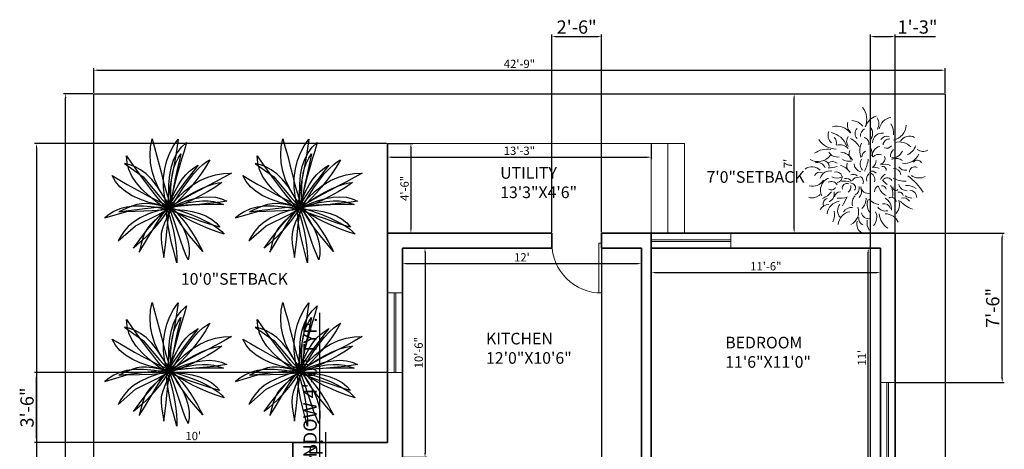
# Model space of a CAD drawing. Units: inches. Extents: x 3394 to 4794, y 965 to 1718.
# Tile 15 of 15: x 4177 to 4770, y 1453 to 1711. Entities that reach past the tile are written whole.
import ezdxf

# ---------------------------------------------------------------- set-up
doc = ezdxf.new("R2010")
doc.units = ezdxf.units.IN
for name, color, linetype, lineweight in [('A-ANNO-DIMS', 2, 'Continuous', 13), ('A-ANNO-TEXT', 7, 'Continuous', 18), ('A-AREA-IDEN', 7, 'Continuous', 18), ('A-DOOR', 4, 'Continuous', 18), ('A-FLOR', 7, 'Continuous', 18), ('A-FLOR-STRS', 7, 'Continuous', 18), ('A-GLAZ', 4, 'Continuous', 18), ('A-WALL', 7, 'Continuous', 35), ('C-PROP', 7, 'Continuous', 25), ('CAY', 94, 'Continuous', 13)]:
    doc.layers.add(name, color=color, linetype=linetype, lineweight=lineweight)
doc.layers.add('DIENHOA', color=3, linetype='Continuous')
doc.styles.add('ATT', font='romans.shx')
doc.styles.get("Standard").update_dxf_attribs({"font": 'arial.ttf'})
doc.dimstyles.new('ISO-25', dxfattribs={"dimtxt": 8, "dimasz": 2.5, "dimexe": 1.25, "dimexo": 0.625, "dimtad": 1, "dimlunit": 3, "dimtxsty": 'Standard', "dimcen": 2.5, "dimadec": 0, "dimazin": 0, "dimtfac": 1, "dimtmove": 0, "dimatfit": 3, "dimfxl": 1, "dimarcsym": 0})

# ---------------------------------------------------------------- blocks, each defined once
blk = doc.blocks.new('*U5')
for p, q in [((0, 0), (0, -6)), ((30, 0), (30, -6))]:
    blk.add_line(p, q)
blk.add_lwpolyline([(0, 0), (0, 30), (1.75, 30), (1.75, 0)], close=True)
blk.add_arc((0, 0), 30, 0, 90)
blk = doc.blocks.new('Cay03_mb')
at = {"layer": 'DIENHOA'}
for p, q in [((79.5, 503.7), (118.6, 555.3)), ((118.6, 555.3), (166.2, 599.1)), ((166.2, 599.1), (142.2, 519.4)), ((48.6, 443.6), (79.5, 503.7)), ((142.2, 519.4), (119, 441.7)), ((-365.2, 390.3), (-414.4, 402.8)), ((-414.4, 402.8), (-240.2, 277.8)), ((-314.9, 371.3), (-365.2, 390.3)), ((-263.5, 343.5), (-314.9, 371.3)), ((9.9, 295.3), (25.5, 374.3)), ((25.5, 374.3), (48.6, 443.6)), ((119, 441.7), (96.7, 365.6)), ((-211.2, 304.6), (-263.5, 343.5)), ((-240.2, 277.8), (-88.4, 94.9)), ((-158, 252.3), (-211.2, 304.6)), ((1.6, 205.7), (9.9, 295.3)), ((75.6, 290.6), (55.7, 216.3)), ((96.7, 365.6), (75.6, 290.6)), ((363.4, 275.4), (436.8, 297.2)), ((436.8, 297.2), (511, 309.6)), ((511, 309.6), (585.9, 313.5)), ((585.9, 313.5), (511.8, 271.4)), ((-104.2, 184.4), (-158, 252.3)), ((-49.6, 98.5), (-104.2, 184.4)), ((0.2, 104.9), (1.6, 205.7)), ((55.7, 216.3), (37.3, 142.1)), ((147, 144.1), (218.5, 199.8)), ((218.5, 199.8), (290.6, 243.2)), ((363.7, 192.9), (290.2, 154.9)), ((290.6, 243.2), (363.4, 275.4)), ((437.6, 231.5), (363.7, 192.9)), ((511.8, 271.4), (437.6, 231.5)), ((-88.4, 94.9), (5.4, -7.8)), ((5.4, -7.8), (-49.6, 98.5)), ((5.4, -7.8), (0.2, 104.9)), ((37.3, 142.1), (20.5, 67.6)), ((75.9, 75.2), (147, 144.1)), ((217.4, 116.6), (145.5, 77.3)), ((290.2, 154.9), (217.4, 116.6)), ((-345, 5.4), (-399.6, -17.1)), ((-298.6, 20.1), (-345, 5.4)), ((-254.7, 27.4), (-298.6, 20.1)), ((-208, 27.8), (-254.7, 27.4)), ((-152.7, 21.7), (-208, 27.8)), ((-83.4, 9.7), (-152.7, 21.7)), ((5.4, -7.8), (-83.4, 9.7)), ((5.4, -7.8), (75.9, 75.2)), ((20.5, 67.6), (5.4, -7.8)), ((74.7, 36.1), (5.4, -7.8)), ((5.4, -7.8), (100.3, 18.4)), ((46.3, 0.9), (5.4, -7.8)), ((96.7, 7.5), (46.3, 0.9)), ((145.5, 77.3), (74.7, 36.1)), ((155, 12.2), (96.7, 7.5)), ((100.3, 18.4), (182.2, 37.2)), ((219.6, 15.4), (155, 12.2)), ((182.2, 37.2), (253, 48.9)), ((289, 17.4), (219.6, 15.4)), ((253, 48.9), (314.6, 54.1)), ((361.6, 18.5), (289, 17.4)), ((314.6, 54.1), (369.2, 53.3)), ((435.8, 18.9), (361.6, 18.5)), ((369.2, 53.3), (418.6, 46.8)), ((418.6, 46.8), (464.9, 35.2)), ((510, 19), (435.8, 18.9)), ((464.9, 35.2), (510, 19)), ((-399.6, -17.1), (-468, -47.9)), ((-468, -47.9), (-375.6, -37.8)), ((-375.6, -37.8), (-295.3, -27.9)), ((-295.3, -27.9), (-225.8, -18.9)), ((-225.8, -18.9), (-165.8, -11.3)), ((-165.8, -11.3), (-114, -5.7)), ((-120.2, -122.1), (-79.8, -79.6)), ((-114, -5.7), (-69, -2.9)), ((-79.8, -79.6), (-45.1, -46.3)), ((-33.2, -69.5), (-74.6, -127.3)), ((-69, -2.9), (-29.6, -3.4)), ((-45.1, -46.3), (-16.5, -22.4)), ((5.4, -7.8), (-33.2, -69.5)), ((-29.6, -3.4), (5.4, -7.8)), ((-16.5, -22.4), (5.4, -7.8)), ((5.4, -7.8), (56.8, -73.3)), ((25.9, -64.4), (5.4, -7.8)), ((5.4, -7.8), (112.8, -40.3)), ((53.5, -41.6), (5.4, -7.8)), ((47, -125.9), (25.9, -64.4)), ((107, -75.7), (53.5, -41.6)), ((56.8, -73.3), (100.4, -139.1)), ((165.5, -109.6), (107, -75.7)), ((112.8, -40.3), (207.5, -73.8)), ((207.5, -73.8), (289.5, -107.6)), ((-216.3, -235.6), (-165.9, -174.1)), ((-165.9, -174.1), (-120.2, -122.1)), ((-117.8, -181.1), (-162.1, -230.9)), ((-74.6, -127.3), (-117.8, -181.1)), ((68.7, -190.6), (47, -125.9)), ((100.4, -139.1), (135.9, -204.3)), ((228.7, -142.8), (165.5, -109.6)), ((296, -174.7), (228.7, -142.8)), ((289.5, -107.6), (359.3, -141.1)), ((367.1, -204.8), (296, -174.7)), ((359.3, -141.1), (416.9, -173.5)), ((416.9, -173.5), (462.6, -204.2)), ((-271, -306.6), (-216.3, -235.6)), ((-162.1, -230.9), (-206.3, -276.5)), ((90.8, -256.6), (68.7, -190.6)), ((113.1, -322.2), (90.8, -256.6)), ((135.9, -204.3), (162.8, -268.3)), ((162.8, -268.3), (181, -330.4)), ((441.6, -232.7), (367.1, -204.8)), ((518.9, -257.7), (441.6, -232.7)), ((462.6, -204.2), (496.5, -232.5)), ((496.5, -232.5), (518.9, -257.7)), ((-329.5, -387.1), (-271, -306.6)), ((-291, -354.7), (-329.5, -387.1)), ((-249.6, -317.8), (-291, -354.7)), ((-206.3, -276.5), (-249.6, -317.8)), ((135.4, -385.6), (113.1, -322.2)), ((181, -330.4), (190, -390)), ((157.6, -445), (135.4, -385.6)), ((179.5, -498.7), (157.6, -445)), ((189.6, -446.3), (179.5, -498.7)), ((190, -390), (189.6, -446.3))]:
    blk.add_line(p, q, dxfattribs=at)
for points in [[(23.7, -5.4), (-41, 82.2), (-91.8, 167.1), (-129.7, 249.5), (-155.6, 329.6), (-170.2, 407.8), (-174.7, 484.2), (-169.8, 559.3), (-156.5, 633.1)], [(-156.5, 633.1), (-132.5, 551.3), (-110.5, 470), (-89.8, 389.2), (-69.6, 309), (-49, 229.4), (-27.1, 150.4), (-3.2, 72.1), (23.7, -5.4)], [(-16.4, -26.7), (-38.3, 80), (-48.9, 178.3), (-48.7, 269), (-38.5, 352.6), (-19.1, 429.7), (9, 501), (44.9, 567.1), (87.9, 628.5)], [(87.9, 628.5), (75.5, 544.2), (61.3, 461.2), (46.1, 379.1), (30.8, 297.8), (16.1, 216.9), (2.9, 136), (-8.3, 54.9), (-16.4, -26.7)], [(-395.6, 473.7), (-347.5, 405.6), (-300.6, 339.5), (-254.3, 275.1), (-208.3, 212.3), (-161.9, 150.9), (-114.8, 90.7), (-66.5, 31.6), (-16.4, -26.7)], [(-16.4, -26.7), (-108.3, 38.6), (-186.9, 101.7), (-252.4, 163.5), (-305.1, 224.4), (-345.4, 285.2), (-373.7, 346.6), (-390.4, 409.2), (-395.6, 473.7)], [(23.7, -5.4), (19.8, 93), (20.3, 177), (25, 248.5), (34, 309.8), (47.3, 362.7), (64.9, 409.3), (86.8, 451.7), (112.9, 491.9)], [(112.9, 491.9), (96, 419.7), (79.5, 347.4), (63.9, 276.5), (50, 208.4), (38.4, 144.8), (29.7, 86.9), (24.6, 36.3), (23.7, -5.4)], [(273.2, 387.3), (227.6, 328.8), (182.3, 270.1), (138.4, 212.3), (97.2, 156.4), (60, 103.4), (27.8, 54.6), (1.9, 10.8), (-16.4, -26.7)], [(-16.4, -26.7), (21.4, 64.2), (57, 140.3), (91.4, 203.3), (125.2, 255.1), (159.5, 297.5), (195, 332.5), (232.7, 361.8), (273.2, 387.3)], [(384.3, 437.5), (342.2, 367.8), (298.1, 301.7), (252.6, 239.4), (206.1, 181.1), (159.4, 127.2), (113, 78), (67.6, 33.6), (23.7, -5.4)], [(23.7, -5.4), (79.9, 91.7), (134.1, 176.2), (185.8, 248.4), (234.3, 308.7), (279, 357.3), (319.3, 394.8), (354.6, 421.4), (384.3, 437.5)], [(-530.5, 289.7), (-458.3, 248.1), (-387.9, 207.8), (-318.9, 168.7), (-250.8, 131.1), (-182.9, 94.8), (-114.9, 59.9), (-46.2, 26.5), (23.7, -5.4)], [(23.7, -5.4), (-87.2, 15.2), (-185, 39.6), (-270.3, 68.2), (-343.7, 101.4), (-405.9, 139.7), (-457.3, 183.5), (-498.7, 233.4), (-530.5, 289.7)], [(496.7, 224), (429.4, 178.4), (361.6, 136.9), (294.1, 99.5), (227.5, 66.1), (162.4, 36.7), (99.7, 11.5), (39.8, -9.7), (-16.4, -26.7)], [(-16.4, -26.7), (75.4, 37.9), (160.1, 91.8), (237.3, 135.7), (306.6, 170), (367.6, 195.4), (419.9, 212.5), (463.1, 221.9), (496.7, 224)], [(-16.4, -26.7), (-134, -4.7), (-235.3, 5.3), (-322, 4.7), (-395.9, -5), (-458.7, -22.3), (-512.3, -45.7), (-558.2, -73.6), (-598.4, -104.7)], [(23.7, -5.4), (99.3, 29.7), (173.2, 57.1), (244.8, 76.7), (313.3, 88.3), (377.9, 91.8), (437.9, 87), (492.7, 73.8), (541.4, 52)], [(541.4, 52), (484.1, 42.9), (421.2, 34.8), (354.4, 27.6), (285.4, 20.9), (216.1, 14.5), (148.2, 8.1), (83.5, 1.6), (23.7, -5.4)], [(-598.4, -104.7), (-392.7, -44.4), (-155, -37.4), (-16.4, -26.7)], [(-471.9, -320.3), (-310.5, -179.3), (-97.7, -73.3), (23.7, -5.4)], [(23.7, -5.4), (-92.3, -34.8), (-188.4, -68.2), (-266.9, -105.1), (-329.9, -144.9), (-379.7, -187), (-418.5, -230.7), (-448.5, -275.3), (-471.9, -320.3)], [(-276.2, -424.4), (-227.3, -345.4), (-185.7, -276.1), (-150, -215.7), (-119.1, -163.8), (-91.5, -119.5), (-66, -82.3), (-41.4, -51.6), (-16.4, -26.7)], [(-16.4, -26.7), (-84.9, -86), (-137, -133.1), (-175.8, -173), (-204.3, -210), (-225.5, -249.1), (-242.5, -294.7), (-258.4, -351.6), (-276.2, -424.4)], [(23.7, -5.4), (-13.6, -87.9), (-41.1, -152.6), (-59.6, -205), (-69.9, -250.7), (-72.8, -295), (-69.2, -343.6), (-59.7, -401.9), (-45.3, -475.5)], [(-45.3, -475.5), (-34.1, -383.2), (-25.4, -302.8), (-18.3, -233.1), (-12, -172.9), (-5.6, -121.2), (2, -76.8), (11.4, -38.5), (23.7, -5.4)], [(76.2, -524.2), (48.8, -428.5), (26.6, -341.7), (9.2, -264.1), (-3.6, -196.1), (-12.3, -138), (-17.1, -90.2), (-18.3, -53), (-16.4, -26.7)], [(-16.4, -26.7), (66.9, -26.6), (145.6, -32.7), (218.8, -44.9), (285.8, -63.1), (345.9, -87.1), (398.4, -116.6), (442.6, -151.6), (477.6, -191.8)], [(477.6, -191.8), (421.8, -176), (361.3, -156.9), (297.6, -135.5), (232.2, -112.6), (166.6, -89.4), (102.3, -66.6), (40.8, -45.4), (-16.4, -26.7)], [(-16.4, -26.7), (8.5, -95.1), (28.5, -163.3), (44.3, -230.6), (56.3, -296.1), (65, -359), (70.9, -418.5), (74.5, -473.9), (76.2, -524.2)], [(316.5, -418.1), (251.4, -342.8), (194.8, -273.3), (146.5, -210.2), (106.3, -153.8), (74.1, -104.7), (49.7, -63.4), (32.9, -30.1), (23.7, -5.4)], [(23.7, -5.4), (74.9, -57.1), (121.8, -110.6), (164.3, -165), (202.7, -219.4), (237, -272.9), (267.3, -324.5), (293.7, -373.2), (316.5, -418.1)]]:
    blk.add_lwpolyline(points, dxfattribs=at)
blk = doc.blocks.new('12PPLT14')
at = {"color": 0, "linetype": 'ByBlock'}
for centre, radius, start, end in [((-0.1625, 0.4338), 0.1552, 335.42338, 39.95274), ((-0.1402, 0.294), 0.1288, 38.23315, 86.42537), ((0.1087, 0.3325), 0.1308, 106.37374, 163.6865), ((-0.0015, 0.3959), 0.0956, 329.29525, 30.70475), ((0.216, 0.3316), 0.1193, 99.66859, 170.39165), ((-0.2571, 0.2399), 0.1351, 34.26616, 106.81595), ((-0.0808, 0.3868), 0.0897, 165.56758, 227.79776), ((-0.0467, 0.3138), 0.0589, 134.27921, 225.72079), ((0.0083, 0.2908), 0.0696, 119.33325, 181.22886), ((-0.0514, 0.3138), 0.0928, 323.30293, 36.69707), ((0.0506, 0.3121), 0.1678, 356.78729, 29.97058), ((0.1909, 0.3893), 0.1338, 281.73118, 357.12575), ((-0.2631, 0.3606), 0.1778, 213.40239, 269.32603), ((-0.2523, 0.2979), 0.0813, 157.25274, 229.50512), ((-0.3428, 0.1468), 0.1777, 20.65225, 77.76096), ((-0.3207, 0.2361), 0.0583, 342.26722, 49.59176), ((-0.1032, 0.2472), 0.0733, 144.90044, 215.09956), ((-0.223, 0.1138), 0.1758, 29.57176, 63.83952), ((-0.0403, 0.2301), 0.0513, 346.72425, 78.69141), ((0.1238, 0.2336), 0.083, 82.99618, 178.26594), ((0.1649, 0.2288), 0.0631, 73.67704, 147.47467), ((0.1827, 0.2139), 0.0534, 85.26504, 175.26709), ((0.3529, 0.1986), 0.0923, 62.48991, 146.60828), ((-0.3406, -0.0039), 0.1849, 80.33595, 125.13865), ((-0.2335, 0.1217), 0.0961, 42.98149, 106.47768), ((-0.071, 0.1405), 0.0841, 159.83302, 213.57269), ((0.103, 0.1659), 0.1687, 157.06159, 198.70067), ((-0.0525, 0.1406), 0.0902, 350.08193, 37.96222), ((0.1187, 0.1278), 0.0788, 101.63592, 188.43663), ((0.1561, 0.2471), 0.0582, 252.24344, 319.67919), ((0.2797, 0.1152), 0.0882, 134.29745, 179.34897), ((0.2662, 0.1039), 0.1379, 44.52266, 106.50759), ((0.2843, 0.2512), 0.1271, 292.72328, 340.80825), ((0.4652, 0.2401), 0.0779, 232.4069, 301.86228), ((-0.4178, 0.2048), 0.1282, 239.72439, 324.07722), ((-0.3739, 0.0341), 0.0511, 2.46695, 87.47281), ((-0.2521, 0.2046), 0.0894, 212.77707, 278.72234), ((-0.2353, 0.0367), 0.1199, 26.17758, 85.19259), ((-0.1543, 0.2003), 0.1209, 241.52868, 278.43473), ((0.0228, 0.0586), 0.0851, 152.04195, 218.82735), ((0.002, 0.1188), 0.05, 112.17477, 182.9374), ((-0.34, 0.1477), 0.3488, 334.29004, 351.88848), ((-0.0111, 0.0925), 0.0832, 308.53514, 354.91362), ((0.094, 0.072), 0.0659, 70.33255, 137.7683), ((0.1017, 0.1024), 0.045, 282.88154, 24.03653), ((0.2042, 0.2053), 0.098, 267.79413, 335.77876), ((0.2424, 0.0217), 0.0815, 51.13973, 117.42715), ((0.3092, 0.1973), 0.1353, 263.34537, 334.18502), ((0.4187, 0.0518), 0.0378, 24.37863, 147.98522), ((-0.468, -0.0701), 0.1027, 47.20219, 124.89917), ((-0.4247, -0.0009), 0.0706, 19.83292, 104.60033), ((-0.2974, 0.0074), 0.0691, 53.51258, 119.74743), ((-0.3432, 0.3083), 0.2855, 272.31468, 287.72191), ((-0.2616, -0.0829), 0.132, 32.23561, 76.03189), ((-0.1183, 0.0408), 0.0581, 157.56093, 237.11283), ((-0.0447, 0.0607), 0.0698, 181.7454, 260.02375), ((0.0563, -0.0634), 0.0921, 62.79175, 99.69781), ((0.1427, -0.0803), 0.1346, 68.72592, 105.24218), ((0.125, 0.0053), 0.0314, 351.8398, 98.09997), ((0.2201, -0.0419), 0.0605, 6.85101, 91.88687), ((0.3159, 0.0688), 0.0649, 214.68942, 281.6662), ((0.3966, -0.0128), 0.0455, 62.41504, 179.56563), ((-0.465, -0.0212), 0.1099, 256.13919, 328.23561), ((-0.4019, -0.0635), 0.0512, 65.26306, 151.643), ((-0.3178, -0.086), 0.0842, 78.28592, 162.92531), ((-0.2877, -0.1629), 0.109, 111.2663, 206.92487), ((-0.2585, 0.0428), 0.1041, 246.13691, 293.86309), ((-0.2636, -0.0603), 0.0501, 19.5336, 107.28809), ((-0.2726, -0.0426), 0.0609, 285.53975, 354.90835), ((-0.1835, -0.1238), 0.059, 37.38554, 100.49906), ((-0.1211, -0.079), 0.0486, 46.81003, 114.24578), ((-0.0834, -0.1038), 0.0488, 74.16701, 155.42913), ((-0.0828, -0.0921), 0.0473, 337.57062, 68.78296), ((0.0687, -0.0762), 0.0776, 139.4669, 188.67411), ((0.0015, -0.0752), 0.0596, 343.19149, 77.68697), ((0.0376, -0.0452), 0.0417, 34.85722, 117.04193), ((0.197, -0.1152), 0.0984, 120.3942, 155.69127), ((0.3403, 0.1226), 0.295, 223.14163, 233.53147), ((0.1639, -0.1068), 0.0471, 29.65158, 136.91476), ((0.3131, 0.1083), 0.1966, 239.63817, 273.34301), ((0.055, -0.4368), 0.4844, 31.85079, 54.27081), ((0.4332, 0.0428), 0.1041, 231.87335, 299.32002), ((-0.3051, -0.1456), 0.0555, 28.56403, 118.62426), ((-0.3049, -0.1199), 0.0412, 237.18619, 328.82945), ((-0.2031, -0.2618), 0.1748, 70.7416, 95.82474), ((-0.1751, -0.1446), 0.0382, 64.59889, 195.07151), ((-0.1983, -0.1346), 0.0584, 307.00435, 10.96098), ((-0.1379, -0.1412), 0.0356, 321.49603, 95.05521), ((-0.1367, -0.1434), 0.0675, 297.46031, 9.45776), ((-0.1261, -0.1768), 0.0743, 318.94457, 21.06007), ((0.0056, -0.1284), 0.0629, 187.60372, 281.90432), ((0.1122, -0.1766), 0.0537, 114.99115, 180.12102), ((0.2021, -0.1018), 0.1155, 193.03502, 246.51688), ((0.1228, -0.1611), 0.0339, 11.25201, 101.31224), ((0.0954, -0.19), 0.1169, 346.83309, 34.71337), ((0.2371, -0.1417), 0.0239, 167.98869, 313.85095), ((0.3301, -0.0984), 0.0696, 193.47929, 272.72308), ((0.3295, -0.2531), 0.1299, 52.41158, 94.15676), ((0.3525, -0.2241), 0.0608, 358.61437, 87.08337), ((-0.4721, -0.1203), 0.1079, 257.32785, 313.21298), ((-0.4582, -0.0549), 0.1957, 293.39465, 321.47421), ((-0.3303, -0.2772), 0.044, 103.55337, 199.89539), ((-0.3545, -0.1945), 0.0737, 295.41723, 13.93701), ((-0.2272, -0.2284), 0.0518, 92.73502, 171.87233), ((-0.2342, -0.0362), 0.1951, 263.47371, 288.55685), ((0.4875, -0.6182), 0.7699, 148.94965, 155.30561), ((-0.0491, -0.2722), 0.0823, 133.29294, 197.24957), ((-0.1342, -0.2328), 0.1218, 315.10673, 1.33197), ((0.0958, -0.2858), 0.1, 154.88084, 226.86789), ((0.0984, -0.1813), 0.1021, 214.34273, 267.49691), ((0.0948, -0.3222), 0.106, 354.64066, 60.41558), ((0.2004, -0.2632), 0.04, 3.12979, 123.69191), ((0.1534, -0.2836), 0.1149, 319.19076, 18.21253), ((0.265, -0.2125), 0.0333, 8.08539, 109.93393), ((0.3002, -0.2876), 0.0597, 31.279, 105.07663), ((0.3711, -0.1347), 0.0953, 234.42972, 271.33095), ((-0.3258, -0.3645), 0.0813, 91.05277, 153.01216), ((-0.2197, -0.3768), 0.1216, 98.93269, 173.56524), ((-0.1666, -0.3361), 0.0858, 141.93744, 222.63897), ((-0.1356, -0.3909), 0.0814, 84.45259, 145.99608), ((-0.1912, -0.3476), 0.1157, 295.67023, 21.36797), ((0.1487, -0.2627), 0.0766, 213.89316, 285.61802), ((0.137, -0.3342), 0.0567, 15.84038, 102.17895), ((0.4504, -0.1006), 0.2342, 221.78679, 251.93539), ((-0.4022, -0.3739), 0.1237, 333.15568, 15.43505), ((-0.1321, -0.4596), 0.1156, 98.85859, 176.18052), ((-0.0165, -0.4023), 0.0586, 172.0702, 247.36769), ((0.0095, -0.3403), 0.0634, 192.71209, 278.21462), ((-0.0287, -0.3897), 0.1058, 317.77354, 24.75223), ((0.2528, -0.3527), 0.1547, 183.87438, 237.37414), ((0.1506, -0.4799), 0.1168, 23.04059, 91.66621), ((-0.0081, -0.4497), 0.0833, 162.96803, 241.48781), ((0.1108, -0.4364), 0.1161, 170.09587, 213.65717)]:
    blk.add_arc(centre, radius, start, end, dxfattribs=at)
at = {"color": 0, "linetype": 'ByBlock', "style": 'ATT'}
for tag, p, flags in [('ITEM', (-1.4111, -3.0457), 3), ('ROOM_NUMBER', (-1.4111, -4.379), 1)]:
    blk.add_attdef(tag, p, '', height=1, dxfattribs=dict(at, flags=flags))
blk = doc.blocks.new('*D32')
at = {"layer": 'A-ANNO-DIMS', "color": 0, "lineweight": -2, "transparency": 16777216}
for p, q in [((4407.27, 1573.06), (4407.27, 1563.11)), ((4551.27, 1573.06), (4551.27, 1563.11)), ((4409.77, 1564.36), (4548.77, 1564.36))]:
    blk.add_line(p, q, dxfattribs=at)
at = {"layer": 'A-ANNO-DIMS', "color": 0, "transparency": 16777216}
for points in [[(4409.77, 1564.78), (4409.77, 1563.95), (4407.27, 1564.36)], [(4548.77, 1564.78), (4548.77, 1563.95), (4551.27, 1564.36)]]:
    blk.add_solid(points, dxfattribs=at)
at = {"layer": 'Defpoints', "color": 0, "transparency": 16777216}
for p in [(4407.27, 1573.68), (4551.27, 1573.68), (4551.27, 1564.36)]:
    blk.add_point(p, dxfattribs=at)
at = {"layer": 'A-ANNO-DIMS', "color": 0, "transparency": 16777216, "insert": (4479.27, 1567.5), "char_height": 5, "attachment_point": 5}
blk.add_mtext("12'", dxfattribs=at)
blk = doc.blocks.new('*D33')
at = {"layer": 'A-ANNO-DIMS', "color": 0, "lineweight": -2, "transparency": 16777216}
for p, q in [((4407.9, 1573.68), (4422.16, 1573.68)), ((4420.91, 1571.18), (4420.91, 1450.18)), ((4407.9, 1447.68), (4422.16, 1447.68))]:
    blk.add_line(p, q, dxfattribs=at)
at = {"layer": 'A-ANNO-DIMS', "color": 0, "transparency": 16777216}
for points in [[(4420.49, 1571.18), (4421.33, 1571.18), (4420.91, 1573.68)], [(4420.49, 1450.18), (4421.33, 1450.18), (4420.91, 1447.68)]]:
    blk.add_solid(points, dxfattribs=at)
at = {"layer": 'Defpoints', "color": 0, "transparency": 16777216}
for p in [(4407.27, 1573.68), (4407.27, 1447.68), (4420.91, 1447.68)]:
    blk.add_point(p, dxfattribs=at)
at = {"layer": 'A-ANNO-DIMS', "color": 0, "transparency": 16777216, "insert": (4417.73, 1510.68), "char_height": 5, "attachment_point": 5, "rotation": 90}
blk.add_mtext('10\'-6"', dxfattribs=at)
blk = doc.blocks.new('*D37')
at = {"layer": 'A-ANNO-DIMS', "color": 0, "lineweight": -2, "transparency": 16777216}
for p, q in [((4642.12, 1666.68), (4644.57, 1666.68)), ((4643.32, 1585.18), (4643.32, 1664.18)), ((4642.12, 1582.68), (4644.57, 1582.68))]:
    blk.add_line(p, q, dxfattribs=at)
at = {"layer": 'A-ANNO-DIMS', "color": 0, "transparency": 16777216}
for points in [[(4642.9, 1664.18), (4643.73, 1664.18), (4643.32, 1666.68)], [(4642.9, 1585.18), (4643.73, 1585.18), (4643.32, 1582.68)]]:
    blk.add_solid(points, dxfattribs=at)
at = {"layer": 'Defpoints', "color": 0, "transparency": 16777216}
for p in [(4641.5, 1666.68), (4643.32, 1666.68), (4641.5, 1582.68)]:
    blk.add_point(p, dxfattribs=at)
at = {"layer": 'A-ANNO-DIMS', "color": 0, "transparency": 16777216, "insert": (4640.19, 1624.68), "char_height": 5, "attachment_point": 5, "rotation": 90}
blk.add_mtext("7'", dxfattribs=at)
blk = doc.blocks.new('*D48')
at = {"layer": 'A-ANNO-DIMS', "color": 0, "lineweight": -2, "transparency": 16777216}
for p, q in [((4694.65, 1573.68), (4686.7, 1573.68)), ((4687.95, 1444.18), (4687.95, 1571.18)), ((4694.65, 1441.68), (4686.7, 1441.68))]:
    blk.add_line(p, q, dxfattribs=at)
at = {"layer": 'A-ANNO-DIMS', "color": 0, "transparency": 16777216}
for points in [[(4687.53, 1571.18), (4688.37, 1571.18), (4687.95, 1573.68)], [(4687.53, 1444.18), (4688.37, 1444.18), (4687.95, 1441.68)]]:
    blk.add_solid(points, dxfattribs=at)
at = {"layer": 'Defpoints', "color": 0, "transparency": 16777216}
for p in [(4687.95, 1573.68), (4695.27, 1573.68), (4695.27, 1441.68)]:
    blk.add_point(p, dxfattribs=at)
at = {"layer": 'A-ANNO-DIMS', "color": 0, "transparency": 16777216, "insert": (4684.81, 1507.68), "char_height": 5, "attachment_point": 5, "rotation": 90}
blk.add_mtext("11'", dxfattribs=at)
blk = doc.blocks.new('*D49')
at = {"layer": 'A-ANNO-DIMS', "color": 0, "lineweight": -2, "transparency": 16777216}
for p, q in [((4557.27, 1573.06), (4557.27, 1557.68)), ((4695.27, 1573.06), (4695.27, 1557.68)), ((4559.77, 1558.93), (4692.77, 1558.93))]:
    blk.add_line(p, q, dxfattribs=at)
at = {"layer": 'A-ANNO-DIMS', "color": 0, "transparency": 16777216}
for points in [[(4559.77, 1559.34), (4559.77, 1558.51), (4557.27, 1558.93)], [(4692.77, 1559.34), (4692.77, 1558.51), (4695.27, 1558.93)]]:
    blk.add_solid(points, dxfattribs=at)
at = {"layer": 'Defpoints', "color": 0, "transparency": 16777216}
for p in [(4557.27, 1573.68), (4695.27, 1573.68), (4695.27, 1558.93)]:
    blk.add_point(p, dxfattribs=at)
at = {"layer": 'A-ANNO-DIMS', "color": 0, "transparency": 16777216, "insert": (4626.27, 1562.11), "char_height": 5, "attachment_point": 5}
blk.add_mtext('11\'-6"', dxfattribs=at)
blk = doc.blocks.new('*D50')
at = {"layer": 'A-ANNO-DIMS', "color": 0, "lineweight": -2, "transparency": 16777216}
for p, q in [((4398.27, 1636.06), (4398.27, 1627.25)), ((4557.27, 1636.06), (4557.27, 1627.25)), ((4400.77, 1628.5), (4554.77, 1628.5))]:
    blk.add_line(p, q, dxfattribs=at)
at = {"layer": 'A-ANNO-DIMS', "color": 0, "transparency": 16777216}
for points in [[(4400.77, 1628.91), (4400.77, 1628.08), (4398.27, 1628.5)], [(4554.77, 1628.91), (4554.77, 1628.08), (4557.27, 1628.5)]]:
    blk.add_solid(points, dxfattribs=at)
at = {"layer": 'Defpoints', "color": 0, "transparency": 16777216}
for p in [(4398.27, 1636.68), (4557.27, 1636.68), (4557.27, 1628.5)]:
    blk.add_point(p, dxfattribs=at)
at = {"layer": 'A-ANNO-DIMS', "color": 0, "transparency": 16777216, "insert": (4477.77, 1631.68), "char_height": 5, "attachment_point": 5}
blk.add_mtext('13\'-3"', dxfattribs=at)
blk = doc.blocks.new('*D51')
at = {"layer": 'A-ANNO-DIMS', "color": 0, "lineweight": -2, "transparency": 16777216}
for p, q in [((4398.9, 1636.68), (4413.65, 1636.68)), ((4412.4, 1634.18), (4412.4, 1585.18)), ((4398.9, 1582.68), (4413.65, 1582.68))]:
    blk.add_line(p, q, dxfattribs=at)
at = {"layer": 'A-ANNO-DIMS', "color": 0, "transparency": 16777216}
for points in [[(4411.98, 1634.18), (4412.82, 1634.18), (4412.4, 1636.68)], [(4411.98, 1585.18), (4412.82, 1585.18), (4412.4, 1582.68)]]:
    blk.add_solid(points, dxfattribs=at)
at = {"layer": 'Defpoints', "color": 0, "transparency": 16777216}
for p in [(4398.27, 1636.68), (4398.27, 1582.68), (4412.4, 1582.68)]:
    blk.add_point(p, dxfattribs=at)
at = {"layer": 'A-ANNO-DIMS', "color": 0, "transparency": 16777216, "insert": (4409.22, 1609.68), "char_height": 5, "attachment_point": 5, "rotation": 90}
blk.add_mtext('4\'-6"', dxfattribs=at)
blk = doc.blocks.new('*D52')
at = {"layer": 'A-ANNO-DIMS', "color": 0, "lineweight": -2, "transparency": 16777216}
for p, q in [((4221.27, 1457.31), (4221.27, 1457.93)), ((4338.77, 1456.68), (4223.77, 1456.68)), ((4341.27, 1456.06), (4341.27, 1455.43))]:
    blk.add_line(p, q, dxfattribs=at)
at = {"layer": 'A-ANNO-DIMS', "color": 0, "transparency": 16777216}
for points in [[(4223.77, 1457.1), (4223.77, 1456.27), (4221.27, 1456.68)], [(4338.77, 1457.1), (4338.77, 1456.27), (4341.27, 1456.68)]]:
    blk.add_solid(points, dxfattribs=at)
at = {"layer": 'Defpoints', "color": 0, "transparency": 16777216}
for p in [(4221.27, 1456.68), (4221.27, 1456.68), (4341.27, 1456.68)]:
    blk.add_point(p, dxfattribs=at)
at = {"layer": 'A-ANNO-DIMS', "color": 0, "transparency": 16777216, "insert": (4281.27, 1459.86), "char_height": 5, "attachment_point": 5}
blk.add_mtext("10'", dxfattribs=at)
blk = doc.blocks.new('*D53')
at = {"layer": 'A-ANNO-DIMS', "color": 0, "lineweight": -2, "transparency": 16777216}
for p, q in [((4220.65, 1666.68), (4203.08, 1666.68)), ((4204.33, 1060.18), (4204.33, 1664.18)), ((4220.65, 1057.68), (4203.08, 1057.68))]:
    blk.add_line(p, q, dxfattribs=at)
at = {"layer": 'A-ANNO-DIMS', "color": 0, "transparency": 16777216}
for points in [[(4203.92, 1664.18), (4204.75, 1664.18), (4204.33, 1666.68)], [(4203.92, 1060.18), (4204.75, 1060.18), (4204.33, 1057.68)]]:
    blk.add_solid(points, dxfattribs=at)
at = {"layer": 'Defpoints', "color": 0, "transparency": 16777216}
for p in [(4204.33, 1666.68), (4221.27, 1666.68), (4221.27, 1057.68)]:
    blk.add_point(p, dxfattribs=at)
at = {"layer": 'A-ANNO-DIMS', "color": 0, "transparency": 16777216, "insert": (4201.15, 1362.18), "char_height": 5, "attachment_point": 5, "rotation": 90}
blk.add_mtext('50\'-9"', dxfattribs=at)
blk = doc.blocks.new('*D54')
at = {"layer": 'A-ANNO-DIMS', "color": 0, "lineweight": -2, "transparency": 16777216}
for p, q in [((4221.27, 1667.31), (4221.27, 1682.11)), ((4223.77, 1680.86), (4731.77, 1680.86)), ((4734.27, 1667.31), (4734.27, 1682.11))]:
    blk.add_line(p, q, dxfattribs=at)
at = {"layer": 'A-ANNO-DIMS', "color": 0, "transparency": 16777216}
for points in [[(4223.77, 1681.27), (4223.77, 1680.44), (4221.27, 1680.86)], [(4731.77, 1681.27), (4731.77, 1680.44), (4734.27, 1680.86)]]:
    blk.add_solid(points, dxfattribs=at)
at = {"layer": 'Defpoints', "color": 0, "transparency": 16777216}
for p in [(4734.27, 1680.86), (4221.27, 1666.68), (4734.27, 1666.68)]:
    blk.add_point(p, dxfattribs=at)
at = {"layer": 'A-ANNO-DIMS', "color": 0, "transparency": 16777216, "insert": (4477.77, 1684.03), "char_height": 5, "attachment_point": 5}
blk.add_mtext('42\'-9"', dxfattribs=at)
blk = doc.blocks.new('WIN-48IN')
for p, q in [((9, 48), (0, 48)), ((4, 0), (4, 48)), ((5, 0), (5, 48)), ((9, 0), (0, 0))]:
    blk.add_line(p, q)
blk = doc.blocks.new('*D62')
at = {"layer": 'A-ANNO-DIMS', "color": 0, "lineweight": -2, "transparency": 16777216}
for p, q in [((4357.47, 1429.68), (4357.47, 1534.67)), ((4350.9, 1429.68), (4358.72, 1429.68)), ((4357.47, 1384.18), (4357.47, 1427.18)), ((4350.9, 1381.68), (4358.72, 1381.68))]:
    blk.add_line(p, q, dxfattribs=at)
at = {"layer": 'A-ANNO-DIMS', "color": 0, "transparency": 16777216}
for points in [[(4357.05, 1427.18), (4357.89, 1427.18), (4357.47, 1429.68)], [(4357.05, 1384.18), (4357.89, 1384.18), (4357.47, 1381.68)]]:
    blk.add_solid(points, dxfattribs=at)
at = {"layer": 'Defpoints', "color": 0, "transparency": 16777216}
for p in [(4350.27, 1429.68), (4357.47, 1429.68), (4350.27, 1381.68)]:
    blk.add_point(p, dxfattribs=at)
at = {"layer": 'A-ANNO-DIMS', "color": 0, "transparency": 16777216, "insert": (4352.71, 1483.42), "char_height": 8, "attachment_point": 5, "rotation": 90}
blk.add_mtext('WINDOW 4\'-0" TYP.', dxfattribs=at)
blk = doc.blocks.new('*D66')
at = {"layer": 'A-ANNO-DIMS', "color": 0, "lineweight": -2, "transparency": 16777216}
for p, q in [((4361.07, 1318.68), (4361.07, 1462.73)), ((4350.9, 1318.68), (4362.32, 1318.68)), ((4361.07, 1249.18), (4361.07, 1316.18)), ((4350.9, 1246.68), (4362.32, 1246.68))]:
    blk.add_line(p, q, dxfattribs=at)
at = {"layer": 'A-ANNO-DIMS', "color": 0, "transparency": 16777216}
for points in [[(4360.65, 1316.18), (4361.49, 1316.18), (4361.07, 1318.68)], [(4360.65, 1249.18), (4361.49, 1249.18), (4361.07, 1246.68)]]:
    blk.add_solid(points, dxfattribs=at)
at = {"layer": 'Defpoints', "color": 0, "transparency": 16777216}
for p in [(4350.27, 1318.68), (4361.07, 1318.68), (4350.27, 1246.68)]:
    blk.add_point(p, dxfattribs=at)
at = {"layer": 'A-ANNO-DIMS', "color": 0, "transparency": 16777216, "insert": (4356.31, 1391.96), "char_height": 8, "attachment_point": 5, "rotation": 90}
blk.add_mtext('LIVING WINDOW 6\'-0" TYP.', dxfattribs=at)
blk = doc.blocks.new('*D107')
at = {"layer": 'A-ANNO-DIMS', "color": 0, "lineweight": -2, "transparency": 16777216}
for p, q in [((4397.65, 1636.68), (4185.57, 1636.68)), ((4186.82, 1634.18), (4186.82, 1120.18)), ((4340.65, 1117.68), (4185.57, 1117.68))]:
    blk.add_line(p, q, dxfattribs=at)
at = {"layer": 'A-ANNO-DIMS', "color": 0, "transparency": 16777216}
for points in [[(4186.4, 1634.18), (4187.24, 1634.18), (4186.82, 1636.68)], [(4186.4, 1120.18), (4187.24, 1120.18), (4186.82, 1117.68)]]:
    blk.add_solid(points, dxfattribs=at)
at = {"layer": 'Defpoints', "color": 0, "transparency": 16777216}
for p in [(4398.27, 1636.68), (4186.82, 1117.68), (4341.27, 1117.68)]:
    blk.add_point(p, dxfattribs=at)
at = {"layer": 'A-ANNO-DIMS', "color": 0, "transparency": 16777216, "insert": (4182.11, 1377.18), "char_height": 8, "attachment_point": 5, "rotation": 90}
blk.add_mtext('43\'-3"', dxfattribs=at)
blk = doc.blocks.new('*D114')
at = {"layer": 'A-ANNO-DIMS', "color": 0, "lineweight": -2, "transparency": 16777216}
for p, q in [((4497.27, 1583.31), (4497.27, 1702.38)), ((4499.77, 1701.13), (4524.77, 1701.13)), ((4527.27, 1583.31), (4527.27, 1702.38))]:
    blk.add_line(p, q, dxfattribs=at)
at = {"layer": 'A-ANNO-DIMS', "color": 0, "transparency": 16777216}
for points in [[(4499.77, 1701.55), (4499.77, 1700.72), (4497.27, 1701.13)], [(4524.77, 1701.55), (4524.77, 1700.72), (4527.27, 1701.13)]]:
    blk.add_solid(points, dxfattribs=at)
at = {"layer": 'Defpoints', "color": 0, "transparency": 16777216}
for p in [(4527.27, 1701.13), (4497.27, 1582.68), (4527.27, 1582.68)]:
    blk.add_point(p, dxfattribs=at)
at = {"layer": 'A-ANNO-DIMS', "color": 0, "transparency": 16777216, "insert": (4512.27, 1705.84), "char_height": 8, "attachment_point": 5}
blk.add_mtext('2\'-6"', dxfattribs=at)
blk = doc.blocks.new('*D117')
at = {"layer": 'A-ANNO-DIMS', "color": 0, "lineweight": -2, "transparency": 16777216}
for p, q in [((4397.65, 1498.68), (4185.57, 1498.68)), ((4186.82, 1459.18), (4186.82, 1496.18)), ((4397.65, 1456.68), (4185.57, 1456.68))]:
    blk.add_line(p, q, dxfattribs=at)
at = {"layer": 'A-ANNO-DIMS', "color": 0, "transparency": 16777216}
for points in [[(4186.4, 1496.18), (4187.24, 1496.18), (4186.82, 1498.68)], [(4186.4, 1459.18), (4187.24, 1459.18), (4186.82, 1456.68)]]:
    blk.add_solid(points, dxfattribs=at)
at = {"layer": 'Defpoints', "color": 0, "transparency": 16777216}
for p in [(4186.82, 1498.68), (4398.27, 1498.68), (4398.27, 1456.68)]:
    blk.add_point(p, dxfattribs=at)
at = {"layer": 'A-ANNO-DIMS', "color": 0, "transparency": 16777216, "insert": (4182.11, 1477.68), "char_height": 8, "attachment_point": 5, "rotation": 90}
blk.add_mtext('3\'-6"', dxfattribs=at)
blk = doc.blocks.new('*D121')
at = {"layer": 'A-ANNO-DIMS', "color": 0, "lineweight": -2, "transparency": 16777216}
for p, q in [((4704.9, 1582.68), (4769.97, 1582.68)), ((4768.72, 1495.18), (4768.72, 1580.18)), ((4704.9, 1492.68), (4769.97, 1492.68))]:
    blk.add_line(p, q, dxfattribs=at)
at = {"layer": 'A-ANNO-DIMS', "color": 0, "transparency": 16777216}
for points in [[(4768.3, 1580.18), (4769.14, 1580.18), (4768.72, 1582.68)], [(4768.3, 1495.18), (4769.14, 1495.18), (4768.72, 1492.68)]]:
    blk.add_solid(points, dxfattribs=at)
at = {"layer": 'Defpoints', "color": 0, "transparency": 16777216}
for p in [(4704.27, 1582.68), (4768.72, 1582.68), (4704.27, 1492.68)]:
    blk.add_point(p, dxfattribs=at)
at = {"layer": 'A-ANNO-DIMS', "color": 0, "transparency": 16777216, "insert": (4764.01, 1537.68), "char_height": 8, "attachment_point": 5, "rotation": 90}
blk.add_mtext('7\'-6"', dxfattribs=at)
blk = doc.blocks.new('*D122')
at = {"layer": 'A-ANNO-DIMS', "color": 0, "lineweight": -2, "transparency": 16777216}
for p, q in [((4689.27, 1199.31), (4689.27, 1702.38)), ((4691.77, 1701.13), (4701.77, 1701.13)), ((4704.27, 1199.31), (4704.27, 1702.38)), ((4704.27, 1701.13), (4728.53, 1701.13))]:
    blk.add_line(p, q, dxfattribs=at)
at = {"layer": 'A-ANNO-DIMS', "color": 0, "transparency": 16777216}
for points in [[(4691.77, 1701.55), (4691.77, 1700.72), (4689.27, 1701.13)], [(4701.77, 1701.55), (4701.77, 1700.72), (4704.27, 1701.13)]]:
    blk.add_solid(points, dxfattribs=at)
at = {"layer": 'Defpoints', "color": 0, "transparency": 16777216}
for p in [(4704.27, 1701.13), (4689.27, 1198.68), (4704.27, 1198.68)]:
    blk.add_point(p, dxfattribs=at)
at = {"layer": 'A-ANNO-DIMS', "color": 0, "transparency": 16777216, "insert": (4717.65, 1705.84), "char_height": 8, "attachment_point": 5}
blk.add_mtext('1\'-3"', dxfattribs=at)
blk = doc.blocks.new('*D128')
at = {"layer": 'A-ANNO-DIMS', "color": 0, "lineweight": -2, "transparency": 16777216}
for p, q in [((4527.27, 1573.06), (4527.27, 987.36)), ((4551.27, 1573.06), (4551.27, 987.36)), ((4529.77, 988.61), (4548.77, 988.61))]:
    blk.add_line(p, q, dxfattribs=at)
at = {"layer": 'A-ANNO-DIMS', "color": 0, "transparency": 16777216}
for points in [[(4529.77, 989.03), (4529.77, 988.2), (4527.27, 988.61)], [(4548.77, 989.03), (4548.77, 988.2), (4551.27, 988.61)]]:
    blk.add_solid(points, dxfattribs=at)
at = {"layer": 'Defpoints', "color": 0, "transparency": 16777216}
for p in [(4527.27, 1573.68), (4551.27, 1573.68), (4551.27, 988.61)]:
    blk.add_point(p, dxfattribs=at)
at = {"layer": 'A-ANNO-DIMS', "color": 0, "transparency": 16777216, "insert": (4539.27, 993.32), "char_height": 8, "attachment_point": 5}
blk.add_mtext('2\'-0"', dxfattribs=at)

msp = doc.modelspace()

# ---------------------------------------------------------------- linework, layer by layer
at = {"layer": 'A-FLOR'}
msp.add_line((4577.27, 1636.682), (4398.27, 1636.682), dxfattribs=at)
at = {"layer": 'A-FLOR-STRS'}
for p, q in [((4557.27, 1582.682), (4557.27, 1636.682)), ((4567.27, 1582.682), (4567.27, 1636.682)), ((4577.27, 1582.682), (4577.27, 1636.682))]:
    msp.add_line(p, q, dxfattribs=at)
at = {"layer": 'A-GLAZ'}
for p, q in [((4557.27, 1578.682), (4605.27, 1578.682)), ((4605.27, 1582.682), (4605.27, 1573.682)), ((4557.27, 1577.682), (4605.27, 1577.682))]:
    msp.add_line(p, q, dxfattribs=at)
at = {"layer": 'A-WALL'}
for p, q in [((4398.27, 1636.682), (4398.27, 1456.682)), ((4398.27, 1582.682), (4497.27, 1582.682)), ((4497.27, 1582.682), (4497.27, 1573.682)), ((4527.27, 1582.682), (4704.27, 1582.682)), ((4527.27, 1582.682), (4527.27, 1573.682)), ((4557.27, 1582.682), (4557.27, 1426.682)), ((4704.27, 1582.682), (4704.27, 1198.682)), ((4407.27, 1573.682), (4497.27, 1573.682)), ((4407.27, 1573.682), (4407.27, 1447.682)), ((4527.27, 1573.682), (4551.27, 1573.682)), ((4551.27, 1573.682), (4551.27, 1426.682)), ((4557.27, 1573.682), (4695.27, 1573.682)), ((4695.27, 1573.682), (4695.27, 1441.682)), ((4341.27, 1117.682), (4341.27, 1456.682)), ((4341.27, 1456.682), (4398.27, 1456.682))]:
    msp.add_line(p, q, dxfattribs=at)
at = {"layer": 'C-PROP'}
for p, q in [((4221.27, 1666.682), (4734.27, 1666.682)), ((4221.27, 1057.682), (4221.27, 1666.682)), ((4734.27, 1666.682), (4734.27, 1057.682))]:
    msp.add_line(p, q, dxfattribs=at)

# ---------------------------------------------------------------- block references
at = {"layer": 'A-DOOR', "rotation": 180.3213350750104}
msp.add_blockref('*U5', (4527.303, 1576.682), dxfattribs=at)
at = {"layer": 'A-GLAZ', "rotation": 180}
msp.add_blockref('WIN-48IN', (4407.27, 1546.683), dxfattribs=at)
at = {"layer": 'A-GLAZ'}
msp.add_blockref('WIN-48IN', (4695.271, 1444.682), dxfattribs=at)
at = {"layer": 'CAY'}
for name, p, xscale, yscale, zscale in [('12PPLT14', (4687.611, 1620.317), 71.57720376410516, 71.57720376410516, 71.57720376410516), ('Cay03_mb', (4266.504, 1598.7), 0.0644925090660235, 0.0644925090660235, 0.0644925090660235), ('Cay03_mb', (4345.264, 1598.7), 0.0644925090660235, 0.0644925090660235, 0.0644925090660235), ('Cay03_mb', (4266.504, 1500.195), 0.0644925090660235, 0.0644925090660235, 0.0644925090660235), ('Cay03_mb', (4345.264, 1500.195), 0.0644925090660235, 0.0644925090660235, 0.0644925090660235)]:
    msp.add_blockref(name, p, dxfattribs=dict(at, xscale=xscale, yscale=yscale, zscale=zscale))

# ---------------------------------------------------------------- texts
at = {"layer": 'A-ANNO-TEXT', "char_height": 7, "attachment_point": 1}
for s, insert in [('{\\fTimes New Roman|b0|i0|c0|p18;7\'0"SETBACK}', (4590.494, 1620.056)), ('{\\fTimes New Roman|b0|i0|c0|p18;10\'0"SETBACK}', (4273.78, 1558.643))]:
    msp.add_mtext_dynamic_manual_height_columns(s, width=61.05572, gutter_width=12.5, heights=[0], dxfattribs=dict(at, insert=insert))
at = {"layer": 'A-AREA-IDEN', "char_height": 7, "attachment_point": 1}
for s, insert in [('{\\fTimes New Roman|b0|i0|c0|p18;UTILITY\\P13\'3"X4\'6"}', (4466.196, 1622.484)), ('{\\fTimes New Roman|b0|i0|c0|p18;KITCHEN\\P12\'0"X10\'6"}', (4457.664, 1522.689)), ('{\\fTimes New Roman|b0|i0|c0|p18;BEDROOM\\P11\'6"X11\'0"}', (4601.815, 1520.29))]:
    msp.add_mtext_dynamic_manual_height_columns(s, width=61.05572, gutter_width=12.5, heights=[0], dxfattribs=dict(at, insert=insert))

# ---------------------------------------------------------------- dimensions: what is measured, and where the dimension line sits
at = {"layer": 'A-ANNO-DIMS'}
for base, p1, p2, override, picture, middle in [((4527.27, 1701.132), (4497.27, 1582.682), (4527.27, 1582.682), {"dimdec": 1, "dimlfac": 1, "dimrnd": 0, "dimzin": 1, "dimdsep": 46, "dimlunit": 4, "dimfrac": 2}, '*D114', (4512.27, 1705.842)), ((4704.27, 1701.132), (4689.27, 1198.682), (4704.27, 1198.682), {"dimdec": 1, "dimlfac": 1, "dimrnd": 0, "dimzin": 1, "dimdsep": 46, "dimlunit": 4, "dimfrac": 2}, '*D122', (4717.652, 1705.845)), ((4734.27, 1680.857), (4221.27, 1666.682), (4734.27, 1666.682), {"dimtxt": 5, "dimclrd": 0, "dimclre": 0, "dimclrt": 0}, '*D54', (4477.77, 1684.035)), ((4557.27, 1628.497), (4398.27, 1636.682), (4557.27, 1636.682), {"dimtxt": 5, "dimclrd": 0, "dimclre": 0, "dimclrt": 0}, '*D50', (4477.77, 1631.677)), ((4551.27, 1564.364), (4407.27, 1573.682), (4551.27, 1573.682), {"dimtxt": 5, "dimclrd": 0, "dimclre": 0, "dimclrt": 0}, '*D32', (4479.27, 1567.499)), ((4551.27, 988.612), (4527.27, 1573.682), (4551.27, 1573.682), {"dimdec": 1, "dimlfac": 1, "dimrnd": 0, "dimzin": 1, "dimdsep": 46, "dimlunit": 4, "dimfrac": 2}, '*D128', (4539.27, 993.322)), ((4695.27, 1558.927), (4557.27, 1573.682), (4695.27, 1573.682), {"dimtxt": 5, "dimclrd": 0, "dimclre": 0, "dimclrt": 0}, '*D49', (4626.27, 1562.105)), ((4221.27, 1456.682), (4341.27, 1456.682), (4221.27, 1456.682), {"dimtxt": 5, "dimclrd": 0, "dimclre": 0, "dimclrt": 0}, '*D52', (4281.27, 1459.86))]:
    dim = msp.add_linear_dim(base=base, p1=p1, p2=p2, dimstyle='ISO-25', override=override, dxfattribs=at)
    dim.commit()
    dim.dimension.update_dxf_attribs({"geometry": picture, "text_midpoint": middle})
for base, p1, p2, override, picture, middle in [((4204.332, 1666.682), (4221.27, 1057.682), (4221.27, 1666.682), {"dimtxt": 5, "dimclrd": 0, "dimclre": 0, "dimclrt": 0}, '*D53', (4201.154, 1362.182)), ((4643.317, 1666.682), (4641.499, 1582.682), (4641.499, 1666.682), {"dimtxt": 5, "dimclrd": 0, "dimclre": 0, "dimclrt": 0}, '*D37', (4640.192, 1624.682)), ((4186.82, 1117.682), (4398.27, 1636.682), (4341.27, 1117.682), {"dimdec": 1, "dimlfac": 1, "dimrnd": 0, "dimzin": 1, "dimdsep": 46, "dimlunit": 4, "dimfrac": 2}, '*D107', (4182.108, 1377.182)), ((4412.399, 1582.682), (4398.27, 1636.682), (4398.27, 1582.682), {"dimtxt": 5, "dimclrd": 0, "dimclre": 0, "dimclrt": 0}, '*D51', (4409.221, 1609.682)), ((4768.72, 1582.682), (4704.27, 1492.682), (4704.27, 1582.682), {"dimdec": 1, "dimlfac": 1, "dimrnd": 0, "dimzin": 1, "dimdsep": 46, "dimlunit": 4, "dimfrac": 2}, '*D121', (4764.011, 1537.682)), ((4420.911, 1447.682), (4407.27, 1573.682), (4407.27, 1447.682), {"dimtxt": 5, "dimclrd": 0, "dimclre": 0, "dimclrt": 0}, '*D33', (4417.733, 1510.682)), ((4687.949, 1573.682), (4695.27, 1441.682), (4695.27, 1573.682), {"dimtxt": 5, "dimclrd": 0, "dimclre": 0, "dimclrt": 0}, '*D48', (4684.814, 1507.682)), ((4186.82, 1498.682), (4398.27, 1456.682), (4398.27, 1498.682), {"dimdec": 1, "dimlfac": 1, "dimrnd": 0, "dimzin": 1, "dimdsep": 46, "dimlunit": 4, "dimfrac": 2}, '*D117', (4182.108, 1477.682))]:
    dim = msp.add_linear_dim(base=base, p1=p1, p2=p2, angle=90, dimstyle='ISO-25', override=override, dxfattribs=at)
    dim.commit()
    dim.dimension.update_dxf_attribs({"geometry": picture, "text_midpoint": middle})
for base, p1, p2, text, picture, middle in [((4357.47, 1429.682), (4350.27, 1381.682), (4350.27, 1429.682), 'WINDOW <> TYP.', '*D62', (4352.706, 1483.424)), ((4361.07, 1318.682), (4350.27, 1246.682), (4350.27, 1318.682), 'LIVING WINDOW <> TYP.', '*D66', (4356.306, 1391.957))]:
    dim = msp.add_linear_dim(base=base, p1=p1, p2=p2, angle=90, text=text, dimstyle='ISO-25', override={"dimdec": 1, "dimlfac": 1, "dimrnd": 0, "dimzin": 1, "dimdsep": 46, "dimlunit": 4, "dimfrac": 2}, dxfattribs=at)
    dim.commit()
    dim.dimension.update_dxf_attribs({"geometry": picture, "text_midpoint": middle})

doc.saveas('drawing.dxf')
